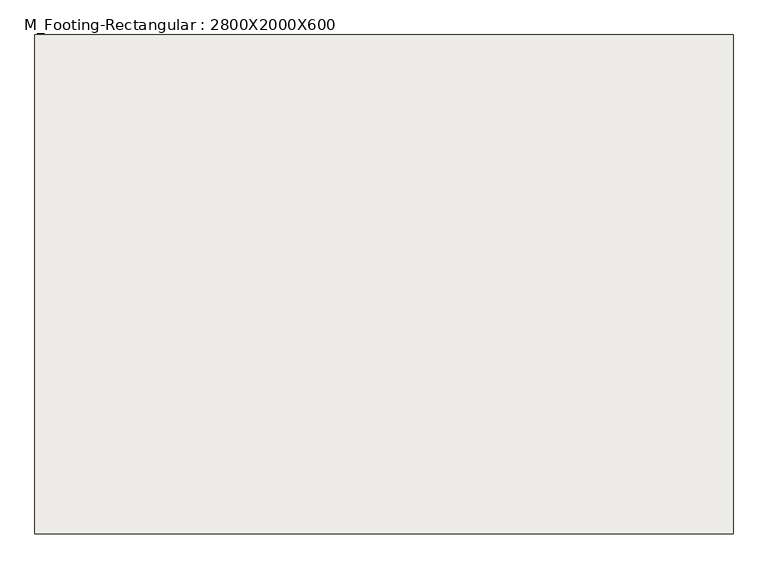
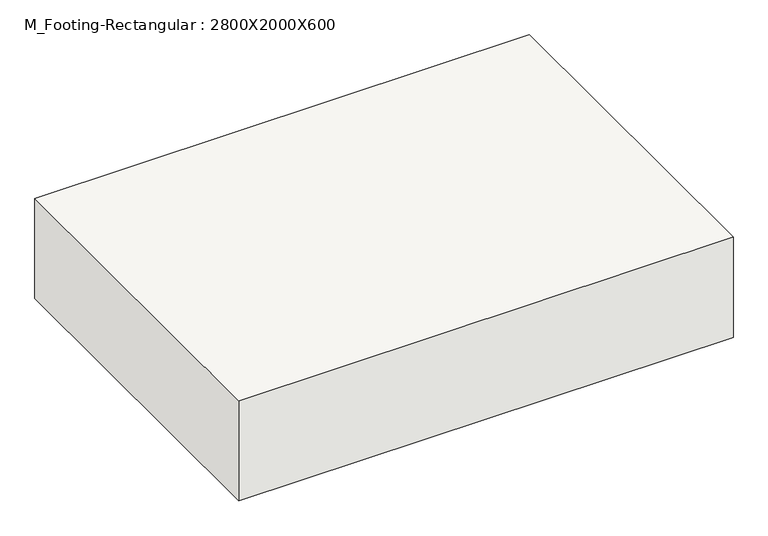
"""IFC4 building model written with IfcOpenShell, lengths in millimetres: slab geometry, M_Footing-Rectangular : 2800X2000X600."""

from ifc_helpers import new_model, si_unit, frame, origin, place, context, project, spatial, polyline, outline, extrude, source, transform, mapped, element, save


def m_footing_rectangular_2800x2000x600_85f03661(model_context):
    return source(origin(), model_context, "Body", "SweptSolid", [
        extrude(outline(polyline([(1400.0, 1000.0), (1400.0, -1000.0), (-1400.0, -1000.0), (-1400.0, 1000.0), (1400.0, 1000.0)])), frame((0.0, 0.0, -600.0), z_axis=(0.0, 0.0, 1.0), x_axis=(1.0, 0.0, 0.0)), (0.0, 0.0, 1.0), 600.0),
    ])


if __name__ == "__main__":
    model = new_model("IFC4")
    model_context = context("Model", 3, world=origin())
    ifc_project = project(units=[si_unit("LENGTHUNIT", "METRE", prefix="MILLI")], contexts=[model_context])
    site = spatial("IfcSite", under=ifc_project)
    building = spatial("IfcBuilding", under=site)
    placement = place(None, origin())
    m_footing_rectangular_2800x2000x600_shape = m_footing_rectangular_2800x2000x600_85f03661(model_context)
    element("IfcSlab", 1, ObjectType="M_Footing-Rectangular : 2800X2000X600", at=placement, inside=building, context=model_context, shape_type="MappedRepresentation", body=[
        mapped(m_footing_rectangular_2800x2000x600_shape, transform((0.0, 0.0, 0.0), x_axis=(1.0, 0.0, 0.0), y_axis=(0.0, 1.0, 0.0), z_axis=(0.0, 0.0, 1.0))),
    ])
    save(model, "model.ifc")

# Revit data of these elements
# Type "M_Footing-Rectangular : 2800X2000X600"
#   Width = 2800 mm
#   Length = 2000 mm
#   Foundation Thickness = 600 mm
#   Structural Material [instance default] = Concrete, Cast-in-Place gray
#   Assembly Code = ""
# Element 1 (IfcSlab, "M_Footing-Rectangular : 2800X2000X600")
#   Structural Material = Concrete, Cast In Situ
#   Materials on its faces: "Concrete, Cast In Situ"
# Materials
#   "Concrete, Cast-in-Place gray": class "Concrete", colour RGB 192 192 192, transparency 0, Description = "Cast-in-place concrete", Cost = 0
#   "Concrete, Cast In Situ": class "Concrete", colour RGB 192 192 192, transparency 0, Description = "physical material", Cost = 0
